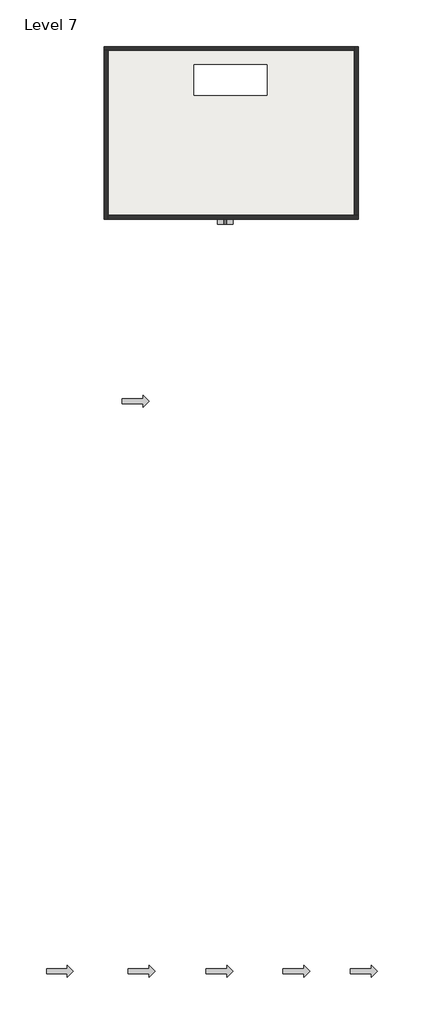
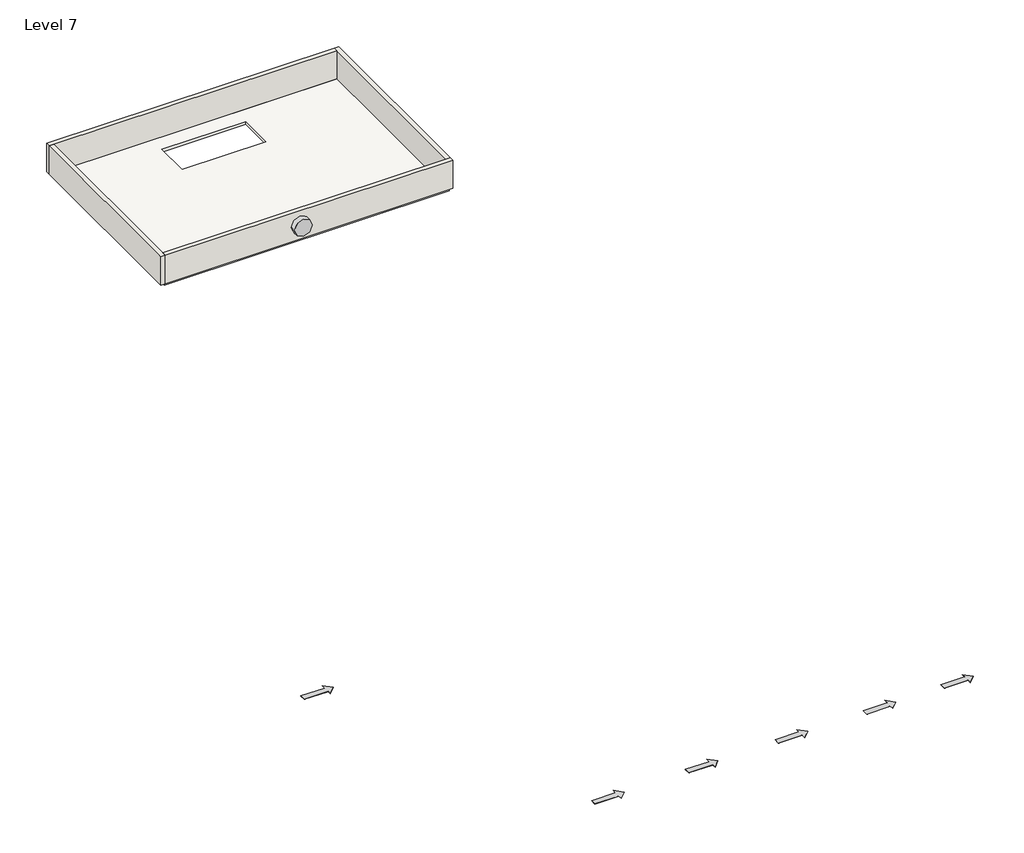
# One storey: 6 geographic elements, 4 walls, 1 proxy, 1 roof.
"""IFC4 building model written with IfcOpenShell, lengths in millimetres."""

from ifc_helpers import new_model, si_unit, frame, origin, place, context, project, spatial, polyline, outline, extrude, faceted_brep, transform, mapped, element, save
from components import generic_models_4_generic_models_4_0bca1b8b, direction_arrows_straight_direction_arrow_straight_a0d3235c

model = new_model("IFC4")

# Units and contexts
model_context = context("Model", 3, world=origin())
ifc_project = project(units=[si_unit("LENGTHUNIT", "METRE", prefix="MILLI")], contexts=[model_context])

# Site, building, storey
site = spatial("IfcSite", under=ifc_project)
building = spatial("IfcBuilding", under=site)
storey = spatial("IfcBuildingStorey", under=building, Name="Level 7", Elevation=16002.0)

# Proxy
placement = place(None, origin())
generic_models_4_generic_models_4_shape = generic_models_4_generic_models_4_0bca1b8b(model_context)
element("IfcBuildingElementProxy", 1, Name="Generic Models 4 : Generic Models 4", ObjectType="Generic Models 4 : Generic Models 4", at=placement, inside=storey, context=model_context, shape_type="MappedRepresentation", body=[
    mapped(generic_models_4_generic_models_4_shape, transform((-304.8, 0.0, 0.0), x_axis=(1.0, 0.0, 0.0), y_axis=(0.0, 1.0, 0.0), z_axis=(0.0, 0.0, 1.0))),
])

# Geographic elements
direction_arrows_straight_direction_arrow_straight_shape = direction_arrows_straight_direction_arrow_straight_a0d3235c(model_context)
element("IfcGeographicElement", 2, ObjectType="Direction Arrows - Straight : Direction Arrow - Straight", at=placement, inside=storey, context=model_context, shape_type="MappedRepresentation", body=[
    mapped(direction_arrows_straight_direction_arrow_straight_shape, transform((-7696.7046642, -13195.4980165, -152.4), x_axis=(0.0, -1.0, 0.0), y_axis=(1.0, 0.0, 0.0), z_axis=(0.0, 0.0, 1.0))),
])
element("IfcGeographicElement", 3, ObjectType="Direction Arrows - Straight : Direction Arrow - Straight", at=placement, inside=storey, context=model_context, shape_type="MappedRepresentation", body=[
    mapped(direction_arrows_straight_direction_arrow_straight_shape, transform((-12137.0126986, -46571.0980165, 16002.0), x_axis=(0.0, -1.0, 0.0), y_axis=(1.0, 0.0, 0.0), z_axis=(0.0, 0.0, 1.0))),
])
element("IfcGeographicElement", 4, ObjectType="Direction Arrows - Straight : Direction Arrow - Straight", at=placement, inside=storey, context=model_context, shape_type="MappedRepresentation", body=[
    mapped(direction_arrows_straight_direction_arrow_straight_shape, transform((-7350.2963491, -46571.0980165, 16002.0), x_axis=(0.0, -1.0, 0.0), y_axis=(1.0, 0.0, 0.0), z_axis=(0.0, 0.0, 1.0))),
])
element("IfcGeographicElement", 5, ObjectType="Direction Arrows - Straight : Direction Arrow - Straight", at=placement, inside=storey, context=model_context, shape_type="MappedRepresentation", body=[
    mapped(direction_arrows_straight_direction_arrow_straight_shape, transform((-2778.2963491, -46571.0980165, 16002.0), x_axis=(0.0, -1.0, 0.0), y_axis=(1.0, 0.0, 0.0), z_axis=(0.0, 0.0, 1.0))),
])
element("IfcGeographicElement", 6, ObjectType="Direction Arrows - Straight : Direction Arrow - Straight", at=placement, inside=storey, context=model_context, shape_type="MappedRepresentation", body=[
    mapped(direction_arrows_straight_direction_arrow_straight_shape, transform((1713.9953358, -46571.0980165, 16002.0), x_axis=(0.0, -1.0, 0.0), y_axis=(1.0, 0.0, 0.0), z_axis=(0.0, 0.0, 1.0))),
])
element("IfcGeographicElement", 7, ObjectType="Direction Arrows - Straight : Direction Arrow - Straight", at=placement, inside=storey, context=model_context, shape_type="MappedRepresentation", body=[
    mapped(direction_arrows_straight_direction_arrow_straight_shape, transform((5676.3953358, -46571.0980165, 16002.0), x_axis=(0.0, -1.0, 0.0), y_axis=(1.0, 0.0, 0.0), z_axis=(0.0, 0.0, 1.0))),
])

# Roof
element("IfcRoof", 8, ObjectType="Generic - 12\"", at=placement, inside=storey, context=model_context, shape_type="SweptSolid", body=[
    extrude(outline(polyline([(6019.2953358, 7335.1167606), (6019.2953358, -2418.4832394), (-8534.9046642, -2418.4832394), (-8534.9046642, 7335.1167606), (6019.2953358, 7335.1167606)]), holes=[polyline([(774.1953358, 6496.9167606), (-3493.0046642, 6496.9167606), (-3493.0046642, 4718.9167606), (774.1953358, 4718.9167606), (774.1953358, 6496.9167606)])]), frame((0.0, 0.0, 15849.6), z_axis=(0.0, 0.0, 1.0), x_axis=(1.0, 0.0, 0.0)), (0.0, 0.0, 1.0), 152.4),
])

# Walls
element("IfcWall", 9, ObjectType="WALL9\"", at=placement, inside=storey, context=model_context, shape_type="Brep", body=[
    faceted_brep([(-8763.5046642, 7335.1167606, 16002.0), (-8534.9046642, 7335.1167606, 16002.0), (5904.9953358, 7335.1167606, 16002.0), (5904.9953358, 7335.1167606, 17526.0), (-8534.9046642, 7335.1167606, 17526.0), (-8763.5046642, 7335.1167606, 17526.0), (-8763.5046642, 7563.7167606, 16002.0), (-8763.5046642, 7563.7167606, 17526.0), (5904.9953358, 7563.7167606, 17526.0), (5904.9953358, 7563.7167606, 16002.0)], [[[0, 1, 2, 3, 4, 5]], [[6, 7, 8, 9]], [[2, 1, 0, 6, 9]], [[5, 4, 3, 8, 7]], [[0, 5, 7, 6]], [[3, 2, 9, 8]]]),
])
element("IfcWall", 10, ObjectType="WALL9\"", at=placement, inside=storey, context=model_context, shape_type="Brep", body=[
    faceted_brep([(-8534.9046642, -2532.7832394, 16002.0), (-8534.9046642, -2304.1832394, 16002.0), (-8534.9046642, 7335.1167606, 16002.0), (-8534.9046642, 7335.1167606, 17526.0), (-8534.9046642, -2304.1832394, 17526.0), (-8534.9046642, -2532.7832394, 17526.0), (-8763.5046642, -2532.7832394, 16002.0), (-8763.5046642, -2532.7832394, 17526.0), (-8763.5046642, 7335.1167606, 17526.0), (-8763.5046642, 7335.1167606, 16002.0)], [[[0, 1, 2, 3, 4, 5]], [[6, 7, 8, 9]], [[2, 1, 0, 6, 9]], [[5, 4, 3, 8, 7]], [[0, 5, 7, 6]], [[3, 2, 9, 8]]]),
])
element("IfcWall", 11, ObjectType="WALL9\"", at=placement, inside=storey, context=model_context, shape_type="Brep", body=[
    faceted_brep([(6133.5953358, -2304.1832394, 16002.0), (5904.9953358, -2304.1832394, 16002.0), (-8534.9046642, -2304.1832394, 16002.0), (-8534.9046642, -2304.1832394, 17526.0), (5904.9953358, -2304.1832394, 17526.0), (6133.5953358, -2304.1832394, 17526.0), (6133.5953358, -2532.7832394, 16002.0), (6133.5953358, -2532.7832394, 17526.0), (-8534.9046642, -2532.7832394, 17526.0), (-8534.9046642, -2532.7832394, 16002.0)], [[[0, 1, 2, 3, 4, 5]], [[6, 7, 8, 9]], [[2, 1, 0, 6, 9]], [[5, 4, 3, 8, 7]], [[0, 5, 7, 6]], [[3, 2, 9, 8]]]),
])
element("IfcWall", 12, ObjectType="WALL9\"", at=placement, inside=storey, context=model_context, shape_type="Brep", body=[
    faceted_brep([(5904.9953358, 7563.7167606, 16002.0), (5904.9953358, 7335.1167606, 16002.0), (5904.9953358, -2304.1832394, 16002.0), (5904.9953358, -2304.1832394, 17526.0), (5904.9953358, 7335.1167606, 17526.0), (5904.9953358, 7563.7167606, 17526.0), (6133.5953358, 7563.7167606, 16002.0), (6133.5953358, 7563.7167606, 17526.0), (6133.5953358, -2304.1832394, 17526.0), (6133.5953358, -2304.1832394, 16002.0)], [[[0, 1, 2, 3, 4, 5]], [[6, 7, 8, 9]], [[2, 1, 0, 6, 9]], [[5, 4, 3, 8, 7]], [[0, 5, 7, 6]], [[3, 2, 9, 8]]]),
])

save(model, "model.ifc")

# Revit data of these elements
# Type "Generic - 12\""
#   Assembly Code = "B1020"
#   Layers, outside or top first: 0' - 6" no material (function 1)
# Type "WALL9\""
#   Assembly Code = "B2010"
#   Layers, outside or top first: 0' - 9" no material (function 1)
# Element 1 (IfcBuildingElementProxy, "Generic Models 4 : Generic Models 4")
#   Phase Created = New Construction
#   Materials on its faces: "Oak Flooring"
# Elements 2, 3, 4, 5, 6, 7 (IfcGeographicElement, "Direction Arrows - Straight : Direction Arrow - Straight")
#   Phase Created = New Construction
#   Materials on its faces: "Paint - White"
# Element 8 (IfcRoof, "Generic - 12\"")
#   built-in parameter 1001705 = 52.5 (stored number, unit not read)
#   built-in parameter 1001701 = -0.5 (stored number, unit not read)
#   built-in parameter 1001710 = 33615
#   Phase Created = New Construction
#   Materials on its faces: "Default Roof"
# Elements 9, 10, 11, 12 (IfcWall, "WALL9\"")
#   Top Offset = 0' - 0"
#   Base Offset = 0' - 0"
#   Unconnected Height = 5' - 0"
#   wall height = 5' - 0"
#   Phase Created = New Construction
#   Base Constraint = Level 7
#   Materials on its faces: "Default Wall"
# Materials
#   "Oak Flooring": class "Wood", colour RGB 216 169 114, transparency 0, Description = "Quercus Rubra", Cost = 0
#   "Paint - White": class "Paint", colour RGB 249 249 249, transparency 0
#   "Default Roof": colour RGB 88 101 114, transparency 0, Cost = 0
#   "Default Wall": colour RGB 128 128 128, transparency 0, Cost = 0
